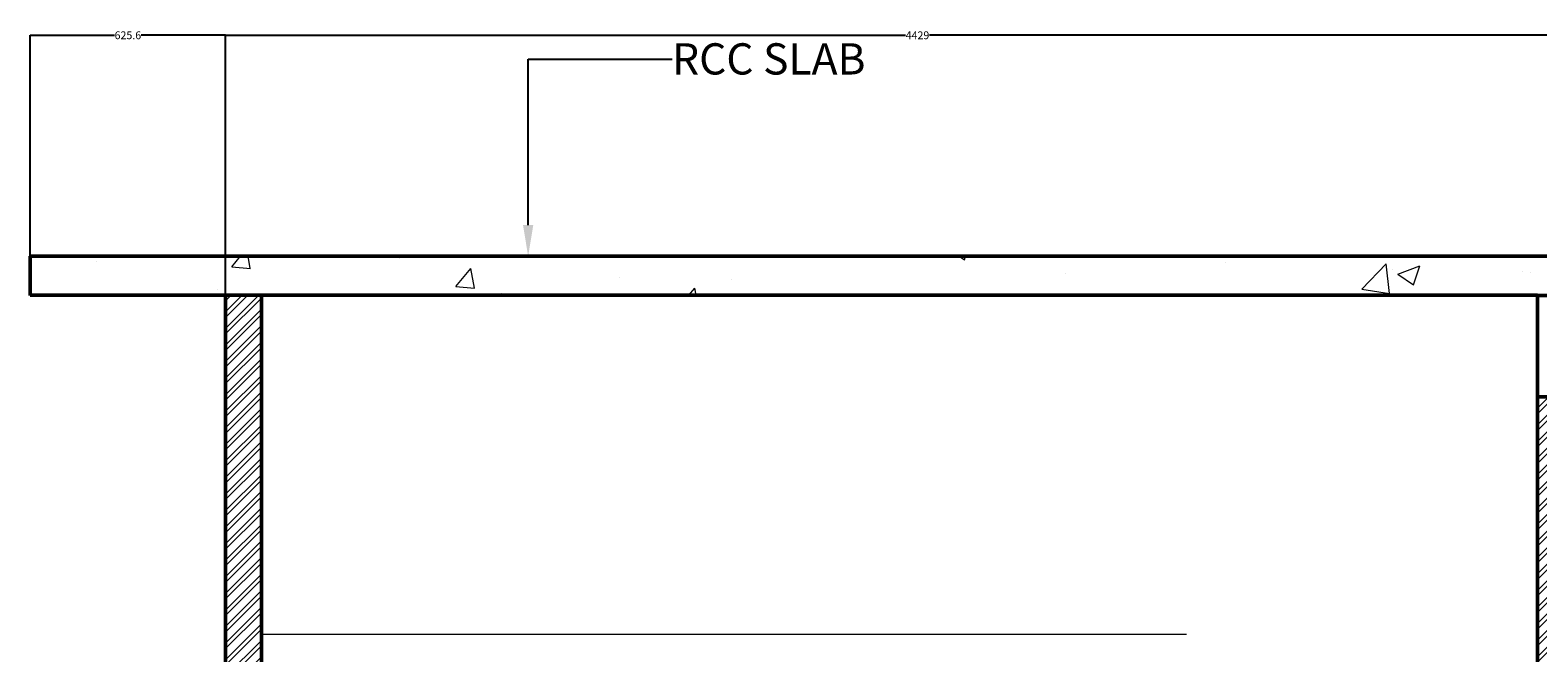
# Model space of a CAD drawing. Units: millimetres. Extents: x 1944 to 29915, y -10550 to 5909.
# Tile 16 of 24: x 12151 to 16977, y 2086 to 4080. Entities that reach past the tile are written whole.
import ezdxf
from ezdxf import colors
from ezdxf.entities.mleader import LeaderData, LeaderLine
from ezdxf.math import Vec2, Vec3

# ---------------------------------------------------------------- set-up
doc = ezdxf.new("R2010")
doc.units = ezdxf.units.MM
doc.header["$MEASUREMENT"] = 0
for name, color, linetype, lineweight in [('A-ANNO-DIMS', 2, 'Continuous', 18), ('A-ANNO-TEXT', 7, 'Continuous', 25), ('A-ELEV', 3, 'Continuous', 18), ('A-WALL', 7, 'Continuous', 50), ('A-WALL-PATT', 8, 'Continuous', 18)]:
    doc.layers.add(name, color=color, linetype=linetype, lineweight=lineweight)
doc.styles.get("Standard").update_dxf_attribs({"font": 'arial.ttf'})
doc.dimstyles.get("Standard").update_dxf_attribs({"dimtxt": 25, "dimasz": 0.18, "dimexe": 0.18, "dimexo": 0.0625, "dimgap": 0.09, "dimtad": 0, "dimtih": 1, "dimtoh": 1, "dimdec": 0, "dimzin": 0, "dimdsep": 46, "dimtxsty": 'Standard', "dimcen": 0.09, "dimadec": 0, "dimazin": 0, "dimtfac": 1, "dimtdec": 0, "dimtofl": 0, "dimtmove": 0, "dimatfit": 3, "dimfxl": 1, "dimtolj": 1, "dimtzin": 0, "dimarcsym": 0})

# ---------------------------------------------------------------- blocks, each defined once
blk = doc.blocks.new('*D60')
at = {"layer": 'A-ANNO-DIMS', "color": 0, "lineweight": -2, "transparency": 16777216}
for p, q in [((12151, 3230.7), (12151, 4063.5)), ((12151.2, 4063.3), (12421.4, 4063.3)), ((12776.4, 4063.3), (12506.1, 4063.3)), ((12776.5, 3230.7), (12776.5, 4063.5))]:
    blk.add_line(p, q, dxfattribs=at)
at = {"layer": 'A-ANNO-DIMS', "color": 0, "transparency": 16777216}
for points in [[(12151.2, 4063.4), (12151.2, 4063.3), (12151, 4063.3)], [(12776.4, 4063.4), (12776.4, 4063.3), (12776.5, 4063.3)]]:
    blk.add_solid(points, dxfattribs=at)
at = {"layer": 'Defpoints', "color": 0, "transparency": 16777216}
for p in [(12776.5, 4063.3), (12151, 3230.7), (12776.5, 3230.7)]:
    blk.add_point(p, dxfattribs=at)
at = {"layer": 'A-ANNO-DIMS', "color": 0, "transparency": 16777216, "insert": (12463.8, 4063.3), "char_height": 25, "attachment_point": 5}
blk.add_mtext('\\A1;625.6', dxfattribs=at)
blk = doc.blocks.new('*D61')
at = {"layer": 'A-ANNO-DIMS', "color": 0, "lineweight": -2, "transparency": 16777216}
for p, q in [((12776.5, 3230.7), (12776.5, 4063.5)), ((12776.7, 4063.3), (14953.2, 4063.3)), ((17205.5, 4063.3), (15029.1, 4063.3)), ((17205.7, 3230.7), (17205.7, 4063.5))]:
    blk.add_line(p, q, dxfattribs=at)
at = {"layer": 'A-ANNO-DIMS', "color": 0, "transparency": 16777216}
for points in [[(12776.7, 4063.4), (12776.7, 4063.3), (12776.5, 4063.3)], [(17205.5, 4063.4), (17205.5, 4063.3), (17205.7, 4063.3)]]:
    blk.add_solid(points, dxfattribs=at)
at = {"layer": 'Defpoints', "color": 0, "transparency": 16777216}
for p in [(17205.7, 4063.3), (12776.5, 3230.7), (17205.7, 3230.7)]:
    blk.add_point(p, dxfattribs=at)
at = {"layer": 'A-ANNO-DIMS', "color": 0, "transparency": 16777216, "insert": (14991.1, 4063.3), "char_height": 25, "attachment_point": 5}
blk.add_mtext('\\A1;4429', dxfattribs=at)

msp = doc.modelspace()

# ---------------------------------------------------------------- hatches: boundary and pattern name
at = {"layer": 'A-WALL-PATT'}
h = msp.add_hatch(dxfattribs=at)
h.set_pattern_fill('AR-CONC', color=256, scale=100)
h.paths.add_polyline_path([(17754.476, 3355.657), (12150.994, 3355.657), (12150.994, 3230.657), (16975.67, 3230.657), (16975.67, 2907.477), (17205.67, 2907.477), (17205.67, 3230.657), (17754.476, 3230.657)])
h = msp.add_hatch(dxfattribs=at)
h.set_pattern_fill('ANSI32', color=256, scale=100)
h.paths.add_polyline_path([(12891.548, 3230.657), (12776.548, 3230.657), (12776.548, 30.837), (12891.548, 30.837)])
h = msp.add_hatch(dxfattribs=at)
h.set_pattern_fill('ANSI32', color=256, scale=100)
h.paths.add_polyline_path([(17205.67, 2905.657), (16975.67, 2905.657), (16975.67, 30.837), (17205.67, 30.837)])

# ---------------------------------------------------------------- linework, layer by layer
at = {"layer": 'A-ELEV'}
msp.add_line((12891.548, 2145.657), (15852.46, 2145.657), dxfattribs=at)
at = {"layer": 'A-WALL'}
for p, q in [((12150.994, 3355.657), (17754.476, 3355.657)), ((12150.994, 3355.657), (12150.994, 3230.477)), ((12150.994, 3230.657), (16975.67, 3230.657)), ((12776.548, 30.837), (12776.548, 3230.657)), ((12891.548, 81.017), (12891.548, 3230.657)), ((16975.67, 81.017), (16975.67, 3230.657)), ((17754.476, 3230.477), (16975.67, 3230.477)), ((17205.67, 2905.657), (16975.67, 2905.657))]:
    msp.add_line(p, q, dxfattribs=at)

# ---------------------------------------------------------------- dimensions: what is measured, and where the dimension line sits
at = {"layer": 'A-ANNO-DIMS'}
for base, p1, p2, override, picture, middle in [((12776.548, 4063.337), (12150.994, 3230.657), (12776.548, 3230.657), {"dimdec": 1, "dimlfac": 1, "dimrnd": 0, "dimzin": 0, "dimdsep": 46, "dimlunit": 2}, '*D60', (12463.771, 4063.337)), ((17205.67, 4063.337), (12776.548, 3230.657), (17205.67, 3230.657), {"dimdec": 0, "dimlfac": 1, "dimrnd": 0, "dimzin": 0, "dimdsep": 46, "dimlunit": 2}, '*D61', (14991.109, 4063.337))]:
    dim = msp.add_linear_dim(base=base, p1=p1, p2=p2, dimstyle='Standard', override=override, dxfattribs=at)
    dim.commit()
    dim.dimension.update_dxf_attribs({"geometry": picture, "text_midpoint": middle})

# ---------------------------------------------------------------- leaders
at = {"layer": 'A-ANNO-TEXT'}
ml = msp.add_multileader_mtext('Standard', dxfattribs=at)
ml.set_content('RCC SLAB ', color=256)
ml.set_leader_properties()
ml.build(insert=Vec2(0, 0))
ml.multileader.update_dxf_attribs({"dogleg_length": 0.36, "arrow_head_size": 100})
ctx = ml.context
ctx.base_point, ctx.char_height, ctx.arrow_head_size, ctx.landing_gap_size, ctx.plane_origin = Vec3(14205.52, 3986.812), 100, 100, 0.09, Vec3(14205.16, 3986.812)
notes = []
notes.append((ctx, [(0, (1, 1, 0), (14205.16, 3986.812), (1, 0), 0.36, [(0, [(13744.97, 3355.657), (13744.97, 3986.812)], 0, [])])]))
ctx.mtext.insert, ctx.mtext.flow_direction = Vec3(14205.61, 4037.665), 5
for ctx, leaders in notes:
    for number, flags, end, landing, length, lines in leaders:
        leader = LeaderData()
        leader.index, (leader.has_last_leader_line, leader.has_dogleg_vector, leader.attachment_direction) = number, flags
        leader.last_leader_point, leader.dogleg_vector, leader.dogleg_length = Vec3(end), Vec3(landing), length
        for number, points, colour, breaks in lines:
            line = LeaderLine()
            line.index, line.vertices, line.color, line.breaks = number, Vec3.list(points), colors.encode_raw_color(colour), breaks
            leader.lines.append(line)
        ctx.leaders.append(leader)

doc.saveas('drawing.dxf')
